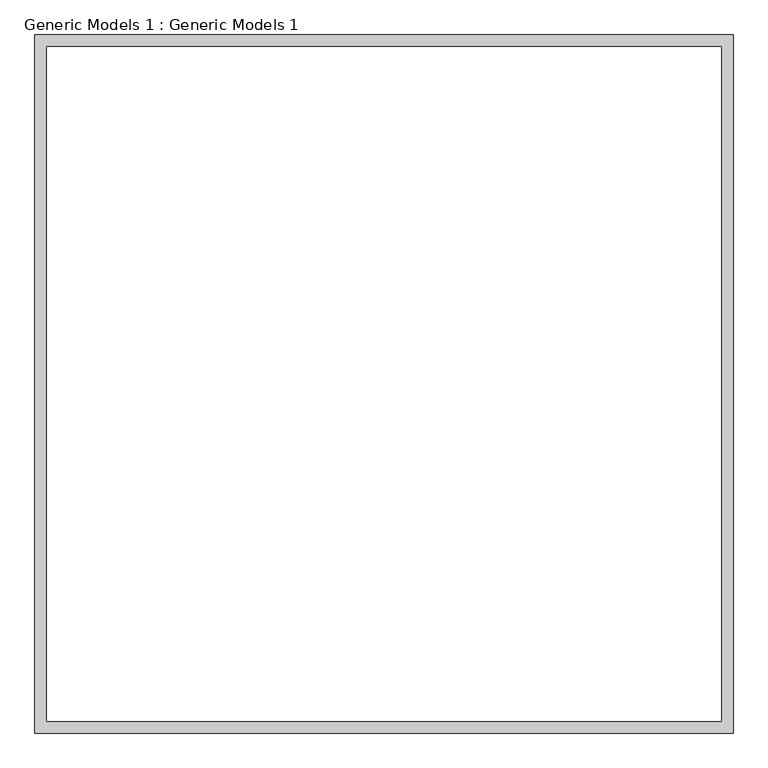
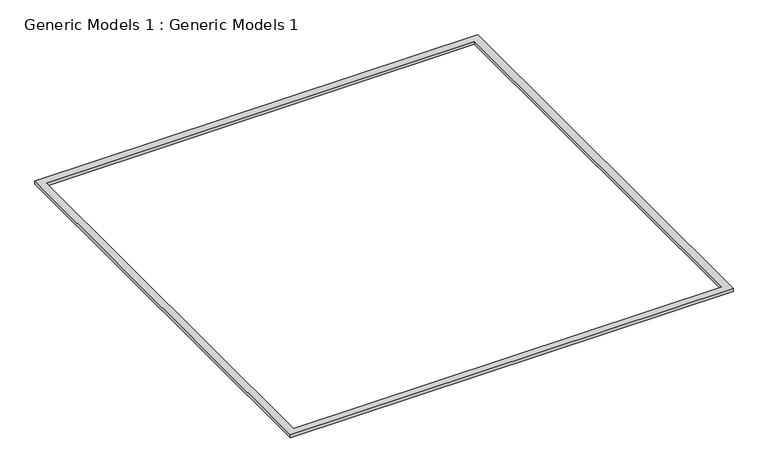
"""IFC4 building model written with IfcOpenShell, lengths in millimetres: proxy geometry, Generic Models 1 : Generic Models 1."""

from ifc_helpers import new_model, si_unit, frame, origin, place, context, project, spatial, polyline, outline, extrude, source, transform, mapped, element, save


def generic_models_1_generic_models_1_aa688ddd(model_context):
    return source(origin(), model_context, "Body", "SweptSolid", [
        extrude(outline(polyline([(-2635.3607439, -3293.8842658), (-2635.3607439, -6341.8842658), (-5683.3607439, -6341.8842658), (-5683.3607439, -3293.8842658), (-2635.3607439, -3293.8842658)]), holes=[polyline([(-2686.1607439, -3344.6842658), (-5632.5607439, -3344.6842658), (-5632.5607439, -6291.0842658), (-2686.1607439, -6291.0842658), (-2686.1607439, -3344.6842658)])]), frame((0.0, 0.0, 3184.6036225), z_axis=(0.0, 0.0, 1.0), x_axis=(1.0, 0.0, 0.0)), (0.0, 0.0, 1.0), 20.9768036),
    ])


if __name__ == "__main__":
    model = new_model("IFC4")
    model_context = context("Model", 3, world=origin())
    ifc_project = project(units=[si_unit("LENGTHUNIT", "METRE", prefix="MILLI")], contexts=[model_context])
    site = spatial("IfcSite", under=ifc_project)
    building = spatial("IfcBuilding", under=site)
    placement = place(None, origin())
    generic_models_1_generic_models_1_shape = generic_models_1_generic_models_1_aa688ddd(model_context)
    element("IfcBuildingElementProxy", 1, Name="Generic Models 1 : Generic Models 1", ObjectType="Generic Models 1 : Generic Models 1", at=placement, inside=building, context=model_context, shape_type="MappedRepresentation", body=[
        mapped(generic_models_1_generic_models_1_shape, transform((0.0, 0.0, 0.0), x_axis=(1.0, 0.0, 0.0), y_axis=(0.0, 1.0, 0.0), z_axis=(0.0, 0.0, 1.0))),
    ])
    save(model, "model.ifc")

# Revit data of these elements
# Element 1 (IfcBuildingElementProxy, "Generic Models 1 : Generic Models 1")
#   Materials on its faces: "Default New Material(1)"
# Materials
#   "Default New Material(1)": class "Generic", colour RGB 120 120 120, transparency 0, Cost = 0
